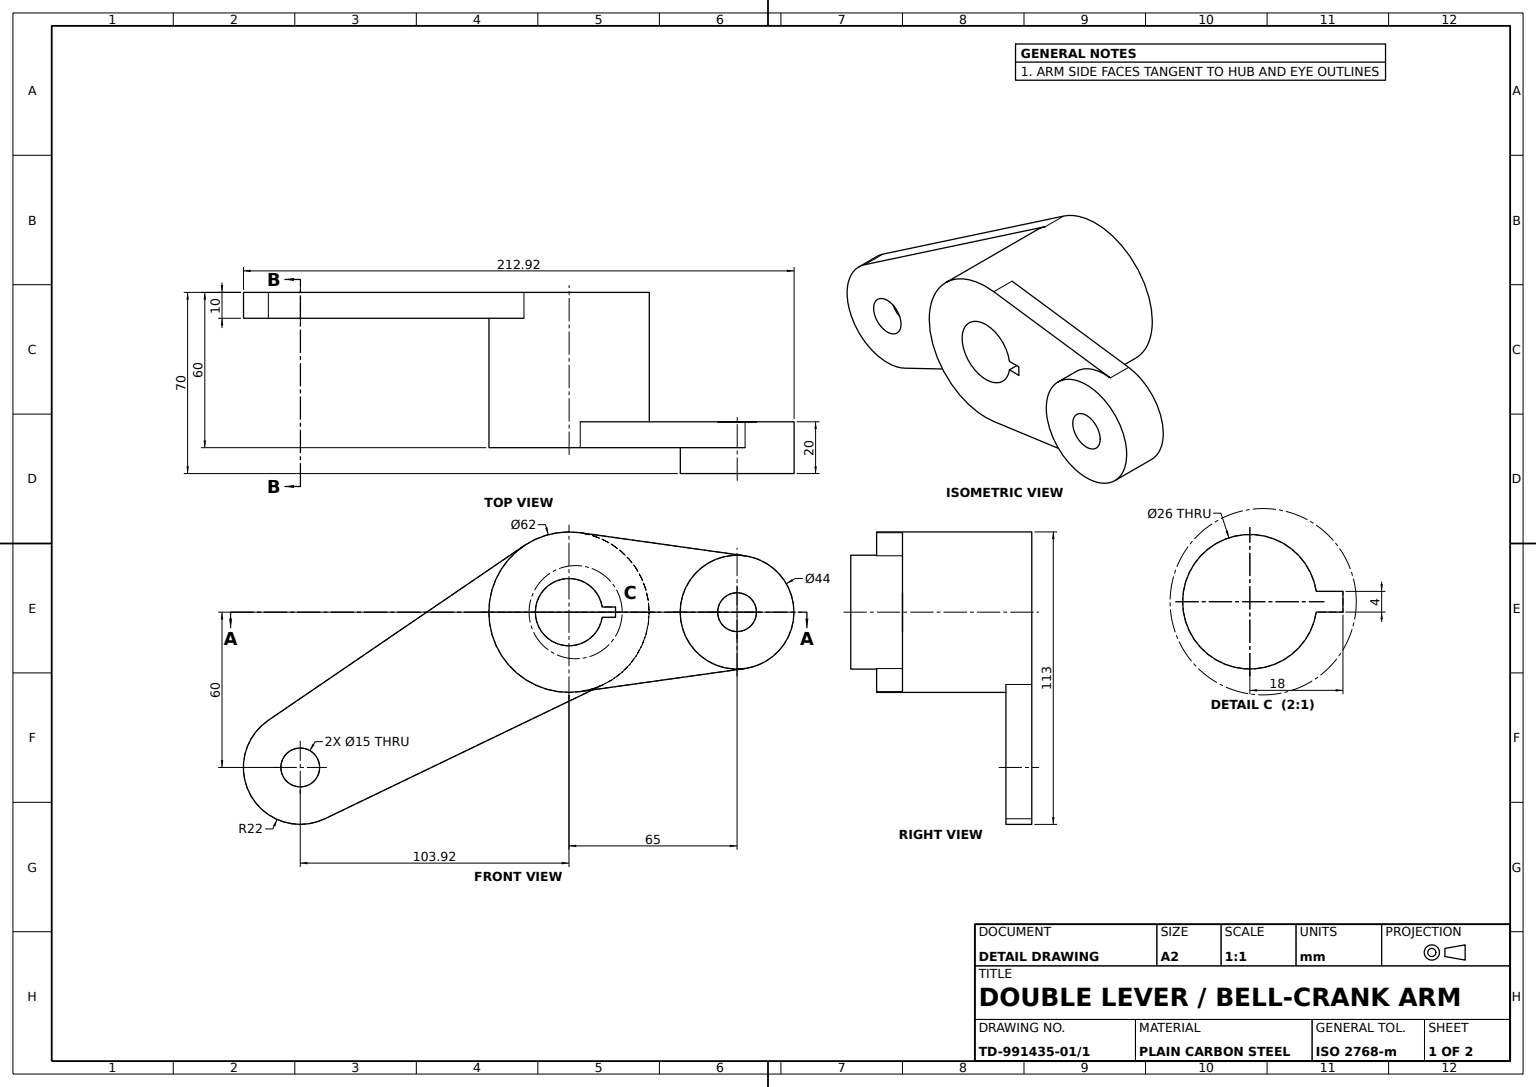
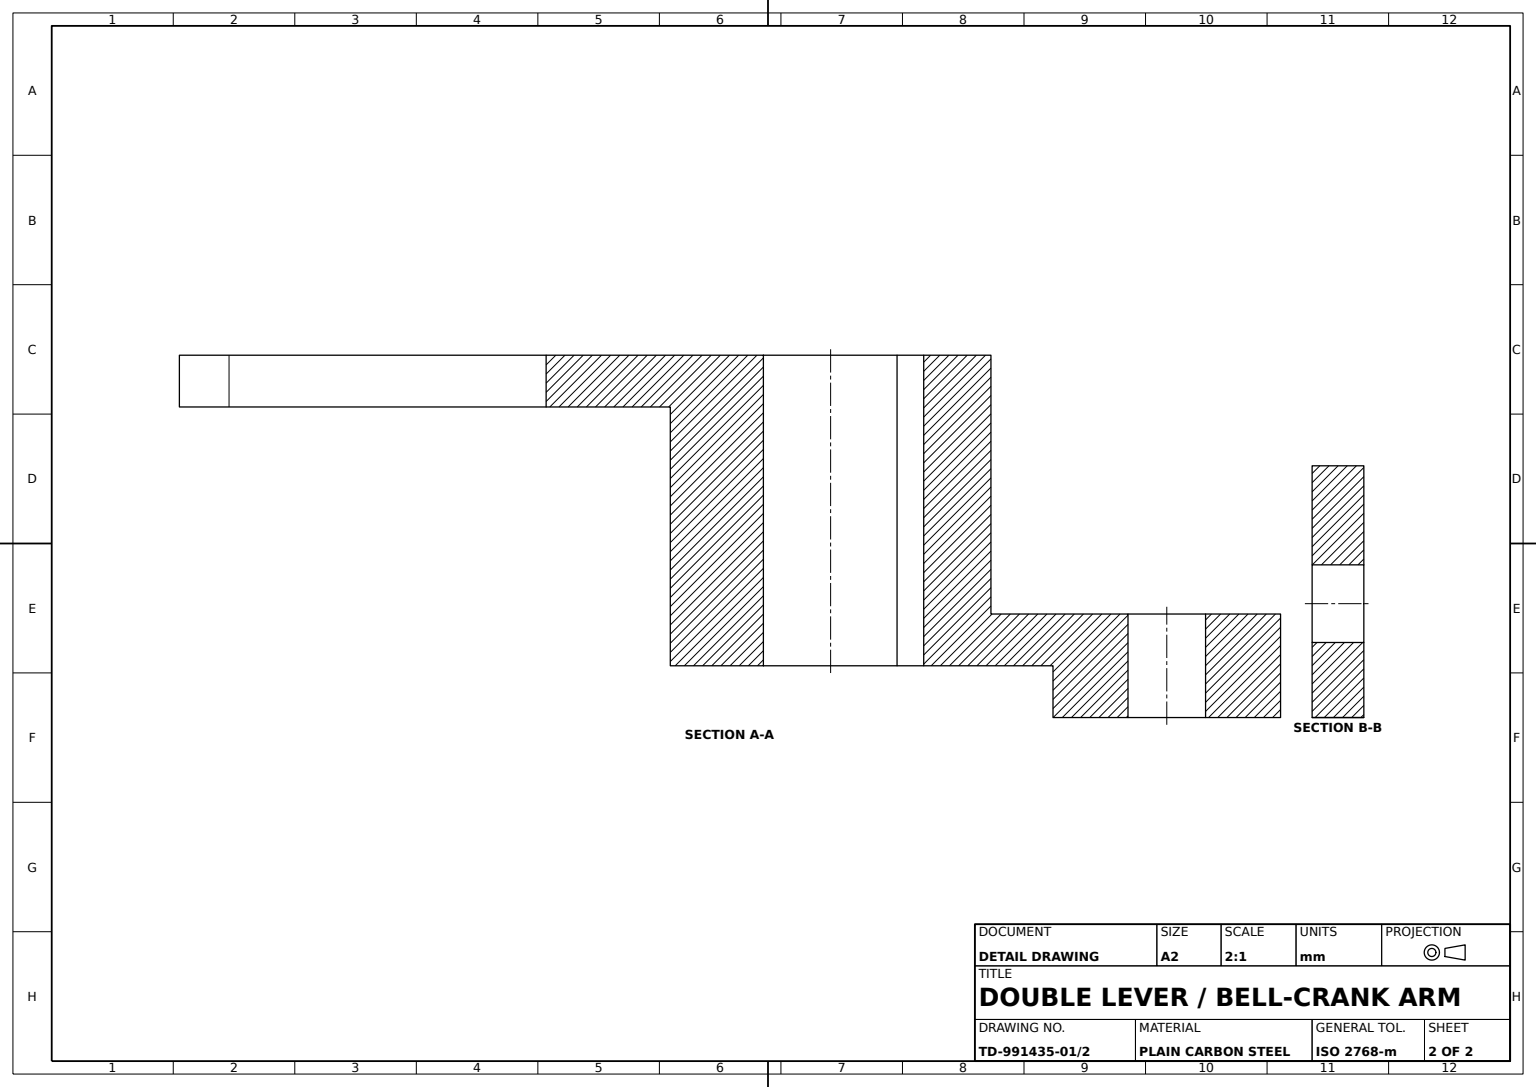
SolidWorks part; units mm, degrees
material "Plain Carbon Steel"
ref_plane "Front Plane" through (0, 0, 0) normal (0, 0, 1) x (1, 0, 0)
ref_plane "Top Plane" through (0, 0, 0) normal (0, 1, 0) x (1, 0, 0)
ref_plane "Right Plane" through (0, 0, 0) normal (1, 0, 0) x (0, 0, -1)
sketch "Arm Plate Profile" plane through (0, 0, 0) normal (0, 0, 1) x (1, 0, 0)
  line L0 (0, 0) -> (65, 0) construction
  line L2 (4.2923, 30.7014) -> (68.0462, 21.7881)
  line L3 (68.0462, -21.7881) -> (4.2923, -30.7014)
  line L5 (12.8452, -2) -> (18, -2) construction
  line L7 (12.8452, 2) -> (18, 2) construction
  line L8 (18, -2) -> (18, 2) construction
  arc A0 (68.0462, -21.7881) -> (68.0462, 21.7881) centre (65, 0) ccw
  arc A1 (4.2923, 30.7014) -> (4.2923, -30.7014) centre (0, 0) ccw
  circle A2 centre (65, 0) radius 22 construction
  arc A3 (12.8452, 2) -> (12.8452, -2) centre (0, 0) ccw construction
  circle A4 centre (0, 0) radius 31 construction
  point P8 (13, 0)
  dimension "D2" = 62
  dimension "D3" = 44
  dimension "D4" = 26
  dimension "D1" = 65
  dimension "D5" = 4
  dimension "D6" = 47
extrude "Arm Plate" add sketch "Arm Plate Profile" against normal blind 10
sketch "Hub Boss Profile" plane through (0, 0, -10) normal (0, 0, -1) x (-1, 0, 0)
  circle A0 centre (-65, 0) radius 22 construction
  circle A1 centre (-65, 0) radius 22
  circle A2 centre (-65, 0) radius 7.5
  dimension "D1" = 15
extrude "Hub Boss" add sketch "Hub Boss Profile" against normal blind 20
sketch "Arm Hole Profile" plane through (0, 0, -10) normal (0, 0, -1) x (-1, 0, 0)
  circle A1 centre (-65, 0) radius 7.5
  circle A2 centre (-65, 0) radius 7.5
  dimension "D1" = 0
extrude "Arm Hole" cut sketch "Arm Hole Profile" against normal through all both and the other way through all
sketch "Hub Housing Profile" plane through (0, 0, -10) normal (0, 0, -1) x (-1, 0, 0)
  line L0 (-12.8452, -2) -> (-18, -2) construction
  line L1 (-12.8452, 2) -> (-18, 2) construction
  line L2 (-18, -2) -> (-18, 2) construction
  line L3 (-12.8452, -2) -> (-18, -2)
  line L4 (-12.8452, 2) -> (-18, 2)
  line L5 (-18, -2) -> (-18, 2)
  arc A0 (-12.8452, -2) -> (-12.8452, 2) centre (0, 0) ccw construction
  circle A1 centre (0, 0) radius 31 construction
  arc A2 (-12.8452, -2) -> (-12.8452, 2) centre (0, 0) ccw
  circle A3 centre (0, 0) radius 31
extrude "Hub Housing" add sketch "Hub Housing Profile" along normal blind 40
sketch "Keyed Bore Profile" plane through (0, 0, -10) normal (0, 0, -1) x (-1, 0, 0)
  line L3 (-18, -2) -> (-12.8452, -2)
  line L4 (-12.8452, 2) -> (-18, 2)
  line L5 (-18, 2) -> (-18, -2)
  line L6 (-18, -2) -> (-12.8452, -2)
  line L7 (-12.8452, 2) -> (-18, 2)
  line L8 (-18, 2) -> (-18, -2)
  arc A1 (-12.8452, -2) -> (-12.8452, 2) centre (0, 0) ccw
  arc A2 (-12.8452, -2) -> (-12.8452, 2) centre (0, 0) ccw
  dimension "D1" = 0
extrude "Keyed Bore" cut sketch "Keyed Bore Profile" against normal through all both and the other way through all
ref_plane "Angled Arm Plane" through (0, 0, -50) normal (0, 0, 1) x (1, 0, 0)
sketch "Angled Arm Profile" plane through (0, 0, -50) normal (0, 0, 1) x (1, 0, 0)
  line L0 (0, 0) -> (-103.923, -60) construction
  line L1 (0, 0) -> (-122.5997, 0) construction
  line L2 (-17.4699, 25.6087) -> (-116.321, -41.8261)
  line L3 (-94.383, -79.8239) -> (13.4428, -27.9337)
  line L4 (18, -2) -> (18, 2) construction
  line L5 (12.8452, -2) -> (18, -2) construction
  line L6 (18, 2) -> (12.8452, 2) construction
  line L7 (18, -2) -> (18, 2)
  line L8 (12.8452, -2) -> (18, -2)
  line L9 (18, 2) -> (12.8452, 2)
  arc A0 (13.4428, -27.9337) -> (-17.4699, 25.6087) centre (0, 0) ccw
  arc A1 (-116.321, -41.8261) -> (-94.383, -79.8239) centre (-103.923, -60) ccw
  circle A2 centre (-103.923, -60) radius 7.5
  arc A3 (12.8452, 2) -> (12.8452, -2) centre (0, 0) ccw construction
  arc A4 (12.8452, 2) -> (12.8452, -2) centre (0, 0) ccw
  dimension "D3" = 44
  dimension "D4" = 15
  dimension "D6" = 62
  dimension "D1" = 120
  dimension "D2" = 30
  dimension "D5" = 31
extrude "Angled Arm Plate" add sketch "Angled Arm Profile" against normal blind 10
